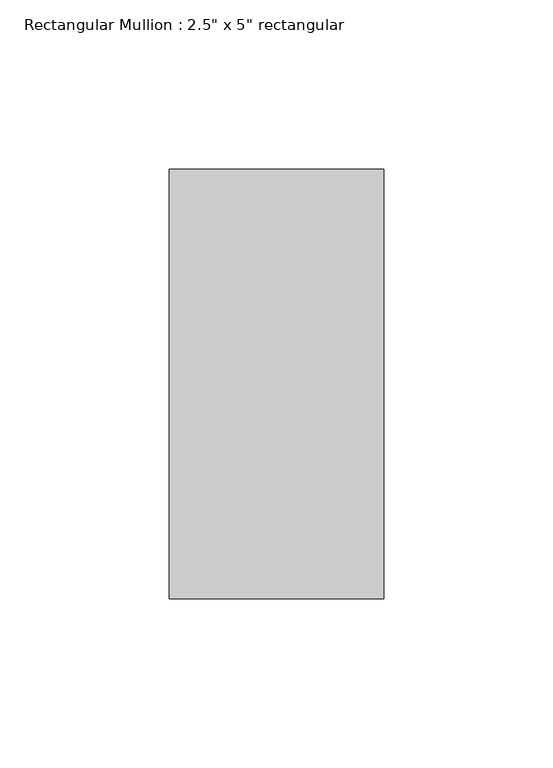
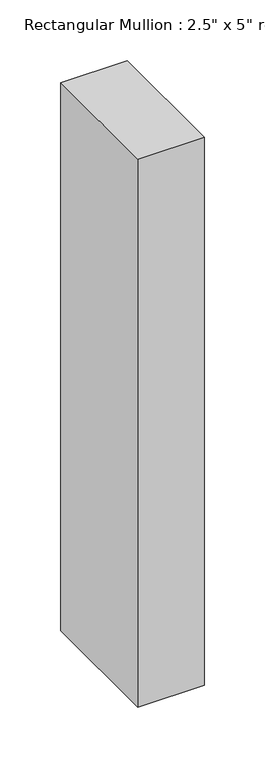
"""IFC4 building model written with IfcOpenShell, lengths in millimetres: member geometry."""

from ifc_helpers import new_model, si_unit, frame, origin, place, context, project, spatial, polyline, outline, extrude, source, transform, mapped, element, save


def member_73c075c8(model_context):
    return source(origin(), model_context, "Body", "SweptSolid", [
        extrude(outline(polyline([(0.0, 63.5), (0.0, -63.5), (-63.5, -63.5), (-63.5, 63.5), (0.0, 63.5)])), frame((0.0, 0.0, -552.45), z_axis=(0.0, 0.0, 1.0), x_axis=(1.0, 0.0, 0.0)), (0.0, 0.0, 1.0), 552.45),
    ])


if __name__ == "__main__":
    model = new_model("IFC4")
    model_context = context("Model", 3, world=origin())
    ifc_project = project(units=[si_unit("LENGTHUNIT", "METRE", prefix="MILLI")], contexts=[model_context])
    site = spatial("IfcSite", under=ifc_project)
    building = spatial("IfcBuilding", under=site)
    placement = place(None, origin())
    member_shape = member_73c075c8(model_context)
    element("IfcMember", 1, ObjectType="Rectangular Mullion : 2.5\" x 5\" rectangular", at=placement, inside=building, context=model_context, shape_type="MappedRepresentation", body=[
        mapped(member_shape, transform((0.0, 0.0, 0.0), x_axis=(1.0, 0.0, 0.0), y_axis=(0.0, 1.0, 0.0), z_axis=(0.0, 0.0, 1.0))),
    ])
    save(model, "model.ifc")

# Revit data of these elements
# Type "Rectangular Mullion : 2.5\" x 5\" rectangular"
#   built-in parameter 1007304 = 0.416667 (stored number, unit not read)
#   built-in parameter 1007301 = 0.104167 (stored number, unit not read)
#   built-in parameter 1007300 = 0.104167 (stored number, unit not read)
